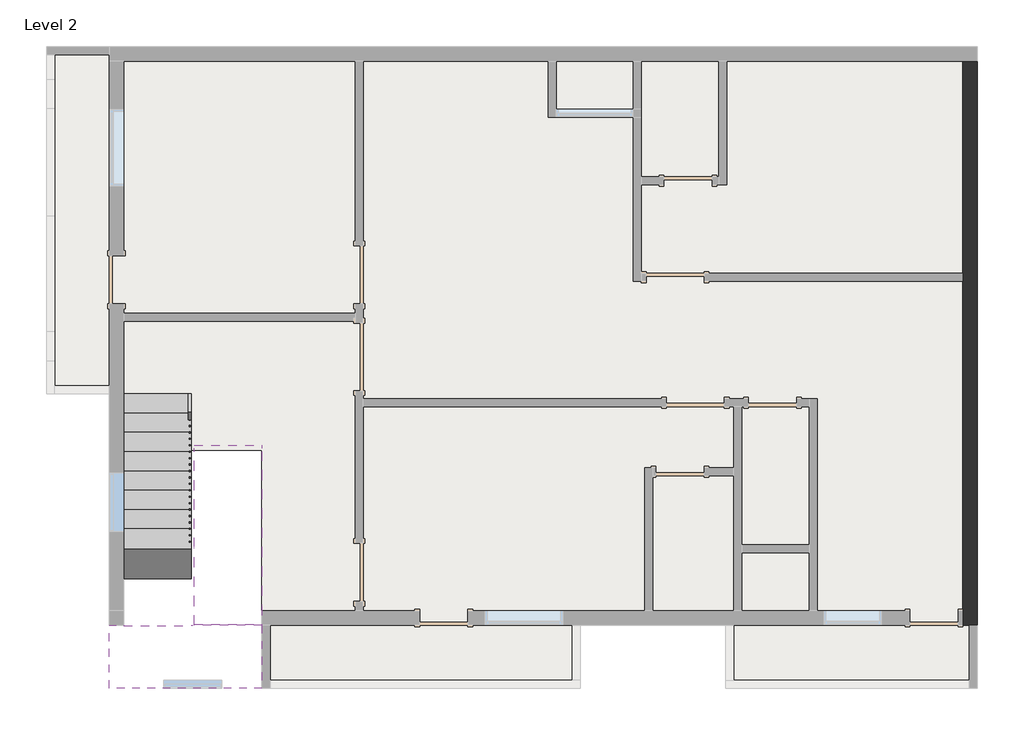
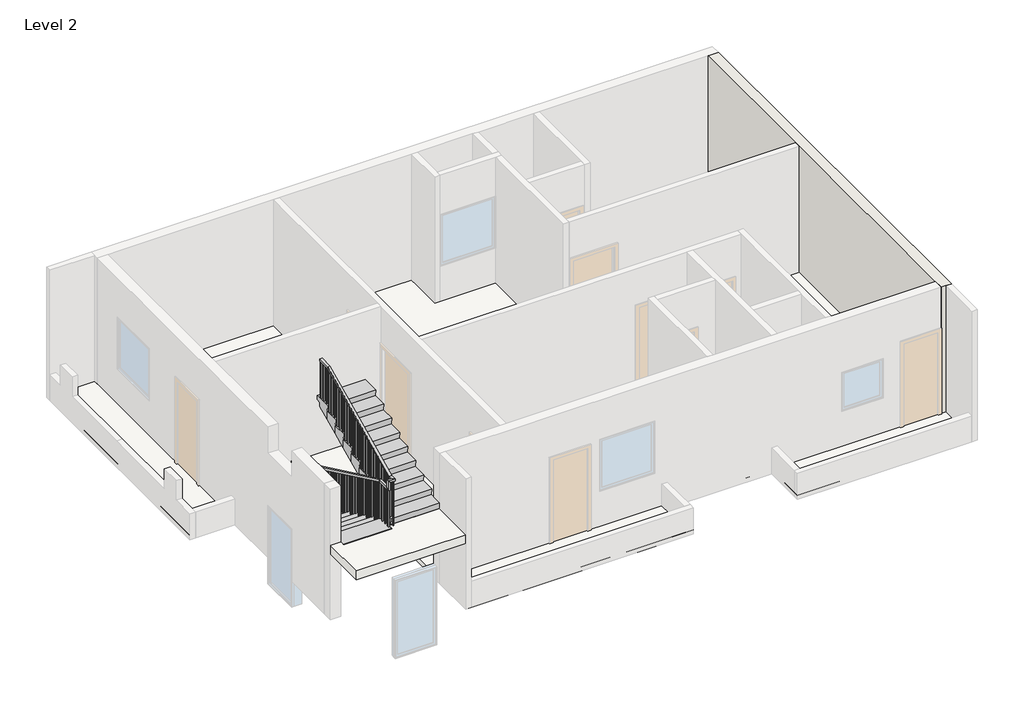
# One storey, part 2 of 2: 2 stair flights, 1 railing, 1 roof, 1 slab, 1 wall.
"""IFC4 building model written with IfcOpenShell, lengths in millimetres."""

from ifc_helpers import new_model, si_unit, frame, origin, place, context, project, spatial, polyline, outline, extrude, faceted_brep, element, save

model = new_model("IFC4")

# Units and contexts
model_context = context("Model", 3, world=origin())
ifc_project = project(units=[si_unit("LENGTHUNIT", "METRE", prefix="MILLI")], contexts=[model_context])

# Site, building, storey
site = spatial("IfcSite", under=ifc_project)
building = spatial("IfcBuilding", under=site)
storey = spatial("IfcBuildingStorey", under=building, Name="Level 2", Elevation=3048.0)

# Railing
placement = place(None, origin())
element("IfcRailing", 1, ObjectType="Handrail - Rectangular", at=placement, inside=storey, context=model_context, shape_type="SolidModel", body=[
    faceted_brep([(-9046.3394758, 7288.0495492, 4107.5428571), (-9046.3394758, 7288.0495492, 4051.2772447), (-9097.1394758, 7288.0495492, 4051.2772447), (-9097.1394758, 7288.0495492, 4107.5428571), (-9046.3394758, 3935.2495492, 5704.1142857), (-9046.3394758, 3923.7717632, 5653.3142857), (-9097.1394758, 3923.7717632, 5653.3142857), (-9097.1394758, 3935.2495492, 5704.1142857), (-9046.3394758, 3630.4495492, 5704.1142857), (-9097.1394758, 3630.4495492, 5704.1142857), (-9097.1394758, 3579.6495492, 5653.3142857), (-9046.3394758, 3579.6495492, 5653.3142857)], [[[0, 1, 2, 3]], [[1, 0, 4, 5]], [[2, 1, 5, 6]], [[3, 2, 6, 7]], [[0, 3, 7, 4]], [[8, 9, 10, 11]], [[5, 4, 8, 11]], [[6, 5, 11, 10]], [[7, 6, 10, 9]], [[4, 7, 9, 8]]]),
    faceted_brep([(-9046.3394758, 3630.4495492, 5704.1142857), (-9046.3394758, 3579.6495492, 5653.3142857), (-9097.1394758, 3579.6495492, 5653.3142857), (-9097.1394758, 3630.4495492, 5704.1142857), (-9046.3394758, 3630.4495492, 5834.7428571), (-9097.1394758, 3630.4495492, 5885.5428571), (-9097.1394758, 3579.6495492, 5885.5428571), (-9046.3394758, 3579.6495492, 5834.7428571)], [[[0, 1, 2, 3]], [[4, 5, 6, 7]], [[1, 0, 4, 7]], [[2, 1, 7, 6]], [[3, 2, 6, 5]], [[0, 3, 5, 4]]]),
    faceted_brep([(-9097.1394758, 3630.4495492, 5885.5428571), (-9046.3394758, 3630.4495492, 5834.7428571), (-9046.3394758, 3579.6495492, 5834.7428571), (-9097.1394758, 3579.6495492, 5885.5428571), (-8995.5394758, 3630.4495492, 5885.5428571), (-8995.5394758, 3630.4495492, 5834.7428571), (-8944.7394758, 3579.6495492, 5834.7428571), (-8944.7394758, 3579.6495492, 5885.5428571), (-8995.5394758, 3706.6495492, 5885.5428571), (-8995.5394758, 3718.1273353, 5834.7428571), (-8944.7394758, 3718.1273353, 5834.7428571), (-8944.7394758, 3706.6495492, 5885.5428571), (-8995.5394758, 6068.8495492, 7010.4), (-8995.5394758, 6080.3273353, 6959.6), (-8944.7394758, 6080.3273353, 6959.6), (-8944.7394758, 6068.8495492, 7010.4), (-8995.5394758, 6373.6495492, 7010.4), (-8944.7394758, 6373.6495492, 7010.4), (-8944.7394758, 6373.6495492, 6959.6), (-8995.5394758, 6373.6495492, 6959.6)], [[[0, 1, 2, 3]], [[1, 0, 4, 5]], [[2, 1, 5, 6]], [[3, 2, 6, 7]], [[0, 3, 7, 4]], [[5, 4, 8, 9]], [[6, 5, 9, 10]], [[7, 6, 10, 11]], [[4, 7, 11, 8]], [[9, 8, 12, 13]], [[10, 9, 13, 14]], [[11, 10, 14, 15]], [[8, 11, 15, 12]], [[16, 17, 18, 19]], [[13, 12, 16, 19]], [[14, 13, 19, 18]], [[15, 14, 18, 17]], [[12, 15, 17, 16]]]),
    extrude(outline(polyline([(-8979.6644758, 6338.7245492), (-8979.6644758, 6357.7745492), (-8960.6144758, 6357.7745492), (-8960.6144758, 6338.7245492), (-8979.6644758, 6338.7245492)])), frame((0.0, 0.0, 6096.0), z_axis=(0.0, 0.0, 1.0), x_axis=(1.0, 0.0, 0.0)), (0.0, 0.0, 1.0), 863.6),
    extrude(outline(polyline([(-8979.6644758, 6237.1245492), (-8979.6644758, 6256.1745492), (-8960.6144758, 6256.1745492), (-8960.6144758, 6237.1245492), (-8979.6644758, 6237.1245492)])), frame((0.0, 0.0, 6096.0), z_axis=(0.0, 0.0, 1.0), x_axis=(1.0, 0.0, 0.0)), (0.0, 0.0, 1.0), 863.6),
    extrude(outline(polyline([(-8979.6644758, 6135.5245492), (-8979.6644758, 6154.5745492), (-8960.6144758, 6154.5745492), (-8960.6144758, 6135.5245492), (-8979.6644758, 6135.5245492)])), frame((0.0, 0.0, 6096.0), z_axis=(0.0, 0.0, 1.0), x_axis=(1.0, 0.0, 0.0)), (0.0, 0.0, 1.0), 863.6),
    extrude(outline(polyline([(6052.9745492, 6946.5748638), (6052.9745492, 5950.8571429), (6033.9245492, 5950.8571429), (6033.9245492, 6937.5034352), (6052.9745492, 6946.5748638)])), frame((-8979.6644758, 0.0, 0.0), z_axis=(1.0, 0.0, 0.0), x_axis=(0.0, 1.0, 0.0)), (0.0, 0.0, 1.0), 19.05),
    extrude(outline(polyline([(5951.3745492, 6898.1939114), (5951.3745492, 5950.8571429), (5932.3245492, 5950.8571429), (5932.3245492, 6889.1224828), (5951.3745492, 6898.1939114)])), frame((-8979.6644758, 0.0, 0.0), z_axis=(1.0, 0.0, 0.0), x_axis=(0.0, 1.0, 0.0)), (0.0, 0.0, 1.0), 19.05),
    extrude(outline(polyline([(5849.7745492, 6849.812959), (5849.7745492, 5950.8571429), (5830.7245492, 5950.8571429), (5830.7245492, 6840.7415305), (5849.7745492, 6849.812959)])), frame((-8979.6644758, 0.0, 0.0), z_axis=(1.0, 0.0, 0.0), x_axis=(0.0, 1.0, 0.0)), (0.0, 0.0, 1.0), 19.05),
    extrude(outline(polyline([(5748.1745492, 6801.4320067), (5748.1745492, 5805.7142857), (5729.1245492, 5805.7142857), (5729.1245492, 6792.3605781), (5748.1745492, 6801.4320067)])), frame((-8979.6644758, 0.0, 0.0), z_axis=(1.0, 0.0, 0.0), x_axis=(0.0, 1.0, 0.0)), (0.0, 0.0, 1.0), 19.05),
    extrude(outline(polyline([(5646.5745492, 6753.0510543), (5646.5745492, 5805.7142857), (5627.5245492, 5805.7142857), (5627.5245492, 6743.9796257), (5646.5745492, 6753.0510543)])), frame((-8979.6644758, 0.0, 0.0), z_axis=(1.0, 0.0, 0.0), x_axis=(0.0, 1.0, 0.0)), (0.0, 0.0, 1.0), 19.05),
    extrude(outline(polyline([(5544.9745492, 6704.6701019), (5544.9745492, 5805.7142857), (5525.9245492, 5805.7142857), (5525.9245492, 6695.5986733), (5544.9745492, 6704.6701019)])), frame((-8979.6644758, 0.0, 0.0), z_axis=(1.0, 0.0, 0.0), x_axis=(0.0, 1.0, 0.0)), (0.0, 0.0, 1.0), 19.05),
    extrude(outline(polyline([(5443.3745492, 6656.2891495), (5443.3745492, 5660.5714286), (5424.3245492, 5660.5714286), (5424.3245492, 6647.2177209), (5443.3745492, 6656.2891495)])), frame((-8979.6644758, 0.0, 0.0), z_axis=(1.0, 0.0, 0.0), x_axis=(0.0, 1.0, 0.0)), (0.0, 0.0, 1.0), 19.05),
    extrude(outline(polyline([(5341.7745492, 6607.9081971), (5341.7745492, 5660.5714286), (5322.7245492, 5660.5714286), (5322.7245492, 6598.8367686), (5341.7745492, 6607.9081971)])), frame((-8979.6644758, 0.0, 0.0), z_axis=(1.0, 0.0, 0.0), x_axis=(0.0, 1.0, 0.0)), (0.0, 0.0, 1.0), 19.05),
    extrude(outline(polyline([(5240.1745492, 6559.5272447), (5240.1745492, 5660.5714286), (5221.1245492, 5660.5714286), (5221.1245492, 6550.4558162), (5240.1745492, 6559.5272447)])), frame((-8979.6644758, 0.0, 0.0), z_axis=(1.0, 0.0, 0.0), x_axis=(0.0, 1.0, 0.0)), (0.0, 0.0, 1.0), 19.05),
    extrude(outline(polyline([(5138.5745492, 6511.1462924), (5138.5745492, 5515.4285714), (5119.5245492, 5515.4285714), (5119.5245492, 6502.0748638), (5138.5745492, 6511.1462924)])), frame((-8979.6644758, 0.0, 0.0), z_axis=(1.0, 0.0, 0.0), x_axis=(0.0, 1.0, 0.0)), (0.0, 0.0, 1.0), 19.05),
    extrude(outline(polyline([(5036.9745492, 6462.76534), (5036.9745492, 5515.4285714), (5017.9245492, 5515.4285714), (5017.9245492, 6453.6939114), (5036.9745492, 6462.76534)])), frame((-8979.6644758, 0.0, 0.0), z_axis=(1.0, 0.0, 0.0), x_axis=(0.0, 1.0, 0.0)), (0.0, 0.0, 1.0), 19.05),
    extrude(outline(polyline([(4935.3745492, 6414.3843876), (4935.3745492, 5515.4285714), (4916.3245492, 5515.4285714), (4916.3245492, 6405.312959), (4935.3745492, 6414.3843876)])), frame((-8979.6644758, 0.0, 0.0), z_axis=(1.0, 0.0, 0.0), x_axis=(0.0, 1.0, 0.0)), (0.0, 0.0, 1.0), 19.05),
    extrude(outline(polyline([(4833.7745492, 6366.0034352), (4833.7745492, 5370.2857143), (4814.7245492, 5370.2857143), (4814.7245492, 6356.9320067), (4833.7745492, 6366.0034352)])), frame((-8979.6644758, 0.0, 0.0), z_axis=(1.0, 0.0, 0.0), x_axis=(0.0, 1.0, 0.0)), (0.0, 0.0, 1.0), 19.05),
    extrude(outline(polyline([(4732.1745492, 6317.6224828), (4732.1745492, 5370.2857143), (4713.1245492, 5370.2857143), (4713.1245492, 6308.5510543), (4732.1745492, 6317.6224828)])), frame((-8979.6644758, 0.0, 0.0), z_axis=(1.0, 0.0, 0.0), x_axis=(0.0, 1.0, 0.0)), (0.0, 0.0, 1.0), 19.05),
    extrude(outline(polyline([(4630.5745492, 6269.2415305), (4630.5745492, 5370.2857143), (4611.5245492, 5370.2857143), (4611.5245492, 6260.1701019), (4630.5745492, 6269.2415305)])), frame((-8979.6644758, 0.0, 0.0), z_axis=(1.0, 0.0, 0.0), x_axis=(0.0, 1.0, 0.0)), (0.0, 0.0, 1.0), 19.05),
    extrude(outline(polyline([(4528.9745492, 6220.8605781), (4528.9745492, 5225.1428571), (4509.9245492, 5225.1428571), (4509.9245492, 6211.7891495), (4528.9745492, 6220.8605781)])), frame((-8979.6644758, 0.0, 0.0), z_axis=(1.0, 0.0, 0.0), x_axis=(0.0, 1.0, 0.0)), (0.0, 0.0, 1.0), 19.05),
    extrude(outline(polyline([(4427.3745492, 6172.4796257), (4427.3745492, 5225.1428571), (4408.3245492, 5225.1428571), (4408.3245492, 6163.4081971), (4427.3745492, 6172.4796257)])), frame((-8979.6644758, 0.0, 0.0), z_axis=(1.0, 0.0, 0.0), x_axis=(0.0, 1.0, 0.0)), (0.0, 0.0, 1.0), 19.05),
    extrude(outline(polyline([(4325.7745492, 6124.0986733), (4325.7745492, 5225.1428571), (4306.7245492, 5225.1428571), (4306.7245492, 6115.0272447), (4325.7745492, 6124.0986733)])), frame((-8979.6644758, 0.0, 0.0), z_axis=(1.0, 0.0, 0.0), x_axis=(0.0, 1.0, 0.0)), (0.0, 0.0, 1.0), 19.05),
    extrude(outline(polyline([(4224.1745492, 6075.7177209), (4224.1745492, 5080.0), (4205.1245492, 5080.0), (4205.1245492, 6066.6462924), (4224.1745492, 6075.7177209)])), frame((-8979.6644758, 0.0, 0.0), z_axis=(1.0, 0.0, 0.0), x_axis=(0.0, 1.0, 0.0)), (0.0, 0.0, 1.0), 19.05),
    extrude(outline(polyline([(4122.5745492, 6027.3367686), (4122.5745492, 5080.0), (4103.5245492, 5080.0), (4103.5245492, 6018.26534), (4122.5745492, 6027.3367686)])), frame((-8979.6644758, 0.0, 0.0), z_axis=(1.0, 0.0, 0.0), x_axis=(0.0, 1.0, 0.0)), (0.0, 0.0, 1.0), 19.05),
    extrude(outline(polyline([(4020.9745492, 5978.9558162), (4020.9745492, 5080.0), (4001.9245492, 5080.0), (4001.9245492, 5969.8843876), (4020.9745492, 5978.9558162)])), frame((-8979.6644758, 0.0, 0.0), z_axis=(1.0, 0.0, 0.0), x_axis=(0.0, 1.0, 0.0)), (0.0, 0.0, 1.0), 19.05),
    extrude(outline(polyline([(3919.3745492, 5930.5748638), (3919.3745492, 4934.8571429), (3900.3245492, 4934.8571429), (3900.3245492, 5921.5034352), (3919.3745492, 5930.5748638)])), frame((-8979.6644758, 0.0, 0.0), z_axis=(1.0, 0.0, 0.0), x_axis=(0.0, 1.0, 0.0)), (0.0, 0.0, 1.0), 19.05),
    extrude(outline(polyline([(3817.7745492, 5882.1939114), (3817.7745492, 4934.8571429), (3798.7245492, 4934.8571429), (3798.7245492, 5873.1224828), (3817.7745492, 5882.1939114)])), frame((-8979.6644758, 0.0, 0.0), z_axis=(1.0, 0.0, 0.0), x_axis=(0.0, 1.0, 0.0)), (0.0, 0.0, 1.0), 19.05),
    extrude(outline(polyline([(3716.1745492, 5833.812959), (3716.1745492, 4934.8571429), (3697.1245492, 4934.8571429), (3697.1245492, 5824.7415305), (3716.1745492, 5833.812959)])), frame((-8979.6644758, 0.0, 0.0), z_axis=(1.0, 0.0, 0.0), x_axis=(0.0, 1.0, 0.0)), (0.0, 0.0, 1.0), 19.05),
    extrude(outline(polyline([(-9062.2144758, 3639.9745492), (-9062.2144758, 3620.9245492), (-9081.2644758, 3620.9245492), (-9081.2644758, 3639.9745492), (-9062.2144758, 3639.9745492)])), frame((0.0, 0.0, 4789.7142857), z_axis=(0.0, 0.0, 1.0), x_axis=(1.0, 0.0, 0.0)), (0.0, 0.0, 1.0), 863.6),
    extrude(outline(polyline([(-9062.2144758, 3741.5745492), (-9062.2144758, 3722.5245492), (-9081.2644758, 3722.5245492), (-9081.2644758, 3741.5745492), (-9062.2144758, 3741.5745492)])), frame((0.0, 0.0, 4789.7142857), z_axis=(0.0, 0.0, 1.0), x_axis=(1.0, 0.0, 0.0)), (0.0, 0.0, 1.0), 863.6),
    extrude(outline(polyline([(-9062.2144758, 3843.1745492), (-9062.2144758, 3824.1245492), (-9081.2644758, 3824.1245492), (-9081.2644758, 3843.1745492), (-9062.2144758, 3843.1745492)])), frame((0.0, 0.0, 4789.7142857), z_axis=(0.0, 0.0, 1.0), x_axis=(1.0, 0.0, 0.0)), (0.0, 0.0, 1.0), 863.6),
    extrude(outline(polyline([(3944.7745492, 5643.312959), (3944.7745492, 4789.7142857), (3925.7245492, 4789.7142857), (3925.7245492, 5652.3843876), (3944.7745492, 5643.312959)])), frame((-9081.2644758, 0.0, 0.0), z_axis=(1.0, 0.0, 0.0), x_axis=(0.0, 1.0, 0.0)), (0.0, 0.0, 1.0), 19.05),
    extrude(outline(polyline([(4046.3745492, 5594.9320067), (4046.3745492, 4644.5714286), (4027.3245492, 4644.5714286), (4027.3245492, 5604.0034352), (4046.3745492, 5594.9320067)])), frame((-9081.2644758, 0.0, 0.0), z_axis=(1.0, 0.0, 0.0), x_axis=(0.0, 1.0, 0.0)), (0.0, 0.0, 1.0), 19.05),
    extrude(outline(polyline([(4147.9745492, 5546.5510543), (4147.9745492, 4644.5714286), (4128.9245492, 4644.5714286), (4128.9245492, 5555.6224828), (4147.9745492, 5546.5510543)])), frame((-9081.2644758, 0.0, 0.0), z_axis=(1.0, 0.0, 0.0), x_axis=(0.0, 1.0, 0.0)), (0.0, 0.0, 1.0), 19.05),
    extrude(outline(polyline([(4249.5745492, 5498.1701019), (4249.5745492, 4644.5714286), (4230.5245492, 4644.5714286), (4230.5245492, 5507.2415305), (4249.5745492, 5498.1701019)])), frame((-9081.2644758, 0.0, 0.0), z_axis=(1.0, 0.0, 0.0), x_axis=(0.0, 1.0, 0.0)), (0.0, 0.0, 1.0), 19.05),
    extrude(outline(polyline([(4351.1745492, 5449.7891495), (4351.1745492, 4499.4285714), (4332.1245492, 4499.4285714), (4332.1245492, 5458.8605781), (4351.1745492, 5449.7891495)])), frame((-9081.2644758, 0.0, 0.0), z_axis=(1.0, 0.0, 0.0), x_axis=(0.0, 1.0, 0.0)), (0.0, 0.0, 1.0), 19.05),
    extrude(outline(polyline([(4452.7745492, 5401.4081971), (4452.7745492, 4499.4285714), (4433.7245492, 4499.4285714), (4433.7245492, 5410.4796257), (4452.7745492, 5401.4081971)])), frame((-9081.2644758, 0.0, 0.0), z_axis=(1.0, 0.0, 0.0), x_axis=(0.0, 1.0, 0.0)), (0.0, 0.0, 1.0), 19.05),
    extrude(outline(polyline([(4554.3745492, 5353.0272447), (4554.3745492, 4499.4285714), (4535.3245492, 4499.4285714), (4535.3245492, 5362.0986733), (4554.3745492, 5353.0272447)])), frame((-9081.2644758, 0.0, 0.0), z_axis=(1.0, 0.0, 0.0), x_axis=(0.0, 1.0, 0.0)), (0.0, 0.0, 1.0), 19.05),
    extrude(outline(polyline([(4655.9745492, 5304.6462924), (4655.9745492, 4354.2857143), (4636.9245492, 4354.2857143), (4636.9245492, 5313.7177209), (4655.9745492, 5304.6462924)])), frame((-9081.2644758, 0.0, 0.0), z_axis=(1.0, 0.0, 0.0), x_axis=(0.0, 1.0, 0.0)), (0.0, 0.0, 1.0), 19.05),
    extrude(outline(polyline([(4757.5745492, 5256.26534), (4757.5745492, 4354.2857143), (4738.5245492, 4354.2857143), (4738.5245492, 5265.3367686), (4757.5745492, 5256.26534)])), frame((-9081.2644758, 0.0, 0.0), z_axis=(1.0, 0.0, 0.0), x_axis=(0.0, 1.0, 0.0)), (0.0, 0.0, 1.0), 19.05),
    extrude(outline(polyline([(4859.1745492, 5207.8843876), (4859.1745492, 4354.2857143), (4840.1245492, 4354.2857143), (4840.1245492, 5216.9558162), (4859.1745492, 5207.8843876)])), frame((-9081.2644758, 0.0, 0.0), z_axis=(1.0, 0.0, 0.0), x_axis=(0.0, 1.0, 0.0)), (0.0, 0.0, 1.0), 19.05),
    extrude(outline(polyline([(4960.7745492, 5159.5034352), (4960.7745492, 4209.1428571), (4941.7245492, 4209.1428571), (4941.7245492, 5168.5748638), (4960.7745492, 5159.5034352)])), frame((-9081.2644758, 0.0, 0.0), z_axis=(1.0, 0.0, 0.0), x_axis=(0.0, 1.0, 0.0)), (0.0, 0.0, 1.0), 19.05),
    extrude(outline(polyline([(5062.3745492, 5111.1224828), (5062.3745492, 4209.1428571), (5043.3245492, 4209.1428571), (5043.3245492, 5120.1939114), (5062.3745492, 5111.1224828)])), frame((-9081.2644758, 0.0, 0.0), z_axis=(1.0, 0.0, 0.0), x_axis=(0.0, 1.0, 0.0)), (0.0, 0.0, 1.0), 19.05),
    extrude(outline(polyline([(5163.9745492, 5062.7415305), (5163.9745492, 4209.1428571), (5144.9245492, 4209.1428571), (5144.9245492, 5071.812959), (5163.9745492, 5062.7415305)])), frame((-9081.2644758, 0.0, 0.0), z_axis=(1.0, 0.0, 0.0), x_axis=(0.0, 1.0, 0.0)), (0.0, 0.0, 1.0), 19.05),
    extrude(outline(polyline([(5265.5745492, 5014.3605781), (5265.5745492, 4064.0), (5246.5245492, 4064.0), (5246.5245492, 5023.4320067), (5265.5745492, 5014.3605781)])), frame((-9081.2644758, 0.0, 0.0), z_axis=(1.0, 0.0, 0.0), x_axis=(0.0, 1.0, 0.0)), (0.0, 0.0, 1.0), 19.05),
    extrude(outline(polyline([(5367.1745492, 4965.9796257), (5367.1745492, 4064.0), (5348.1245492, 4064.0), (5348.1245492, 4975.0510543), (5367.1745492, 4965.9796257)])), frame((-9081.2644758, 0.0, 0.0), z_axis=(1.0, 0.0, 0.0), x_axis=(0.0, 1.0, 0.0)), (0.0, 0.0, 1.0), 19.05),
    extrude(outline(polyline([(5468.7745492, 4917.5986733), (5468.7745492, 4064.0), (5449.7245492, 4064.0), (5449.7245492, 4926.6701019), (5468.7745492, 4917.5986733)])), frame((-9081.2644758, 0.0, 0.0), z_axis=(1.0, 0.0, 0.0), x_axis=(0.0, 1.0, 0.0)), (0.0, 0.0, 1.0), 19.05),
    extrude(outline(polyline([(5570.3745492, 4869.2177209), (5570.3745492, 3918.8571429), (5551.3245492, 3918.8571429), (5551.3245492, 4878.2891495), (5570.3745492, 4869.2177209)])), frame((-9081.2644758, 0.0, 0.0), z_axis=(1.0, 0.0, 0.0), x_axis=(0.0, 1.0, 0.0)), (0.0, 0.0, 1.0), 19.05),
    extrude(outline(polyline([(5671.9745492, 4820.8367686), (5671.9745492, 3918.8571429), (5652.9245492, 3918.8571429), (5652.9245492, 4829.9081971), (5671.9745492, 4820.8367686)])), frame((-9081.2644758, 0.0, 0.0), z_axis=(1.0, 0.0, 0.0), x_axis=(0.0, 1.0, 0.0)), (0.0, 0.0, 1.0), 19.05),
    extrude(outline(polyline([(5773.5745492, 4772.4558162), (5773.5745492, 3918.8571429), (5754.5245492, 3918.8571429), (5754.5245492, 4781.5272447), (5773.5745492, 4772.4558162)])), frame((-9081.2644758, 0.0, 0.0), z_axis=(1.0, 0.0, 0.0), x_axis=(0.0, 1.0, 0.0)), (0.0, 0.0, 1.0), 19.05),
    extrude(outline(polyline([(5875.1745492, 4724.0748638), (5875.1745492, 3773.7142857), (5856.1245492, 3773.7142857), (5856.1245492, 4733.1462924), (5875.1745492, 4724.0748638)])), frame((-9081.2644758, 0.0, 0.0), z_axis=(1.0, 0.0, 0.0), x_axis=(0.0, 1.0, 0.0)), (0.0, 0.0, 1.0), 19.05),
    extrude(outline(polyline([(5976.7745492, 4675.6939114), (5976.7745492, 3773.7142857), (5957.7245492, 3773.7142857), (5957.7245492, 4684.76534), (5976.7745492, 4675.6939114)])), frame((-9081.2644758, 0.0, 0.0), z_axis=(1.0, 0.0, 0.0), x_axis=(0.0, 1.0, 0.0)), (0.0, 0.0, 1.0), 19.05),
    extrude(outline(polyline([(6078.3745492, 4627.312959), (6078.3745492, 3773.7142857), (6059.3245492, 3773.7142857), (6059.3245492, 4636.3843876), (6078.3745492, 4627.312959)])), frame((-9081.2644758, 0.0, 0.0), z_axis=(1.0, 0.0, 0.0), x_axis=(0.0, 1.0, 0.0)), (0.0, 0.0, 1.0), 19.05),
    extrude(outline(polyline([(6179.9745492, 4578.9320067), (6179.9745492, 3628.5714286), (6160.9245492, 3628.5714286), (6160.9245492, 4588.0034352), (6179.9745492, 4578.9320067)])), frame((-9081.2644758, 0.0, 0.0), z_axis=(1.0, 0.0, 0.0), x_axis=(0.0, 1.0, 0.0)), (0.0, 0.0, 1.0), 19.05),
    extrude(outline(polyline([(6281.5745492, 4530.5510543), (6281.5745492, 3628.5714286), (6262.5245492, 3628.5714286), (6262.5245492, 4539.6224828), (6281.5745492, 4530.5510543)])), frame((-9081.2644758, 0.0, 0.0), z_axis=(1.0, 0.0, 0.0), x_axis=(0.0, 1.0, 0.0)), (0.0, 0.0, 1.0), 19.05),
    extrude(outline(polyline([(6383.1745492, 4482.1701019), (6383.1745492, 3628.5714286), (6364.1245492, 3628.5714286), (6364.1245492, 4491.2415305), (6383.1745492, 4482.1701019)])), frame((-9081.2644758, 0.0, 0.0), z_axis=(1.0, 0.0, 0.0), x_axis=(0.0, 1.0, 0.0)), (0.0, 0.0, 1.0), 19.05),
    extrude(outline(polyline([(6484.7745492, 4433.7891495), (6484.7745492, 3483.4285714), (6465.7245492, 3483.4285714), (6465.7245492, 4442.8605781), (6484.7745492, 4433.7891495)])), frame((-9081.2644758, 0.0, 0.0), z_axis=(1.0, 0.0, 0.0), x_axis=(0.0, 1.0, 0.0)), (0.0, 0.0, 1.0), 19.05),
    extrude(outline(polyline([(6586.3745492, 4385.4081971), (6586.3745492, 3483.4285714), (6567.3245492, 3483.4285714), (6567.3245492, 4394.4796257), (6586.3745492, 4385.4081971)])), frame((-9081.2644758, 0.0, 0.0), z_axis=(1.0, 0.0, 0.0), x_axis=(0.0, 1.0, 0.0)), (0.0, 0.0, 1.0), 19.05),
    extrude(outline(polyline([(6687.9745492, 4337.0272447), (6687.9745492, 3483.4285714), (6668.9245492, 3483.4285714), (6668.9245492, 4346.0986733), (6687.9745492, 4337.0272447)])), frame((-9081.2644758, 0.0, 0.0), z_axis=(1.0, 0.0, 0.0), x_axis=(0.0, 1.0, 0.0)), (0.0, 0.0, 1.0), 19.05),
    extrude(outline(polyline([(6789.5745492, 4288.6462924), (6789.5745492, 3338.2857143), (6770.5245492, 3338.2857143), (6770.5245492, 4297.7177209), (6789.5745492, 4288.6462924)])), frame((-9081.2644758, 0.0, 0.0), z_axis=(1.0, 0.0, 0.0), x_axis=(0.0, 1.0, 0.0)), (0.0, 0.0, 1.0), 19.05),
    extrude(outline(polyline([(6891.1745492, 4240.26534), (6891.1745492, 3338.2857143), (6872.1245492, 3338.2857143), (6872.1245492, 4249.3367686), (6891.1745492, 4240.26534)])), frame((-9081.2644758, 0.0, 0.0), z_axis=(1.0, 0.0, 0.0), x_axis=(0.0, 1.0, 0.0)), (0.0, 0.0, 1.0), 19.05),
    extrude(outline(polyline([(6992.7745492, 4191.8843876), (6992.7745492, 3338.2857143), (6973.7245492, 3338.2857143), (6973.7245492, 4200.9558162), (6992.7745492, 4191.8843876)])), frame((-9081.2644758, 0.0, 0.0), z_axis=(1.0, 0.0, 0.0), x_axis=(0.0, 1.0, 0.0)), (0.0, 0.0, 1.0), 19.05),
    extrude(outline(polyline([(7094.3745492, 4143.5034352), (7094.3745492, 3193.1428571), (7075.3245492, 3193.1428571), (7075.3245492, 4152.5748638), (7094.3745492, 4143.5034352)])), frame((-9081.2644758, 0.0, 0.0), z_axis=(1.0, 0.0, 0.0), x_axis=(0.0, 1.0, 0.0)), (0.0, 0.0, 1.0), 19.05),
    extrude(outline(polyline([(7195.9745492, 4095.1224828), (7195.9745492, 3193.1428571), (7176.9245492, 3193.1428571), (7176.9245492, 4104.1939114), (7195.9745492, 4095.1224828)])), frame((-9081.2644758, 0.0, 0.0), z_axis=(1.0, 0.0, 0.0), x_axis=(0.0, 1.0, 0.0)), (0.0, 0.0, 1.0), 19.05),
    extrude(outline(polyline([(-8979.6644758, 3614.5745492), (-8960.6144758, 3614.5745492), (-8960.6144758, 3595.5245492), (-8979.6644758, 3595.5245492), (-8979.6644758, 3614.5745492)])), frame((0.0, 0.0, 4789.7142857), z_axis=(0.0, 0.0, 1.0), x_axis=(1.0, 0.0, 0.0)), (0.0, 0.0, 1.0), 1045.0285714),
    extrude(outline(polyline([(-9062.2144758, 3614.5745492), (-9062.2144758, 3595.5245492), (-9081.2644758, 3595.5245492), (-9081.2644758, 3614.5745492), (-9062.2144758, 3614.5745492)])), frame((0.0, 0.0, 4789.7142857), z_axis=(0.0, 0.0, 1.0), x_axis=(1.0, 0.0, 0.0)), (0.0, 0.0, 1.0), 863.6),
    extrude(outline(polyline([(-8979.6644758, 6354.5995492), (-8979.6644758, 6373.6495492), (-8960.6144758, 6373.6495492), (-8960.6144758, 6354.5995492), (-8979.6644758, 6354.5995492)])), frame((0.0, 0.0, 6096.0), z_axis=(0.0, 0.0, 1.0), x_axis=(1.0, 0.0, 0.0)), (0.0, 0.0, 1.0), 863.6),
    extrude(outline(polyline([(7288.0495492, 4051.2772447), (7288.0495492, 3193.1428571), (7268.9995492, 3193.1428571), (7268.9995492, 4060.3486733), (7288.0495492, 4051.2772447)])), frame((-9081.2644758, 0.0, 0.0), z_axis=(1.0, 0.0, 0.0), x_axis=(0.0, 1.0, 0.0)), (0.0, 0.0, 1.0), 19.05),
])

# Roof
element("IfcRoof", 2, ObjectType="Generic - 4\"", at=placement, inside=storey, context=model_context, shape_type="SweptSolid", body=[
    extrude(outline(polyline([(3374.2605242, 2639.8495492), (-600.8394758, 2639.8495492), (-600.8394758, 3630.4495492), (-2899.5394758, 3630.4495492), (-2899.5394758, 2639.8495492), (-7928.7394758, 2639.8495492), (-7928.7394758, 6399.0495492), (-9046.3394758, 6399.0495492), (-9046.3394758, 7288.0495492), (-11332.3394758, 7288.0495492), (-11332.3394758, 12774.4495492), (3374.2605242, 12774.4495492), (3374.2605242, 2639.8495492)])), frame((0.0, 0.0, 3048.0), z_axis=(0.0, 0.0, 1.0), x_axis=(1.0, 0.0, 0.0)), (0.0, 0.0, 1.0), 101.6),
])

# Slab
element("IfcSlab", 3, ObjectType="8\" Thickness", at=placement, inside=storey, context=model_context, shape_type="Brep", body=[
    faceted_brep([(-10341.7394758, 3630.4495492, 4789.7142857), (-10341.7394758, 2639.8495492, 4789.7142857), (-7928.7394758, 2639.8495492, 4789.7142857), (-7928.7394758, 3630.4495492, 4789.7142857), (-7928.7394758, 3649.4995492, 4789.7142857), (-8995.5394758, 3649.4995492, 4789.7142857), (-8995.5394758, 3630.4495492, 4789.7142857), (-9044.7519758, 3630.4495492, 4789.7142857), (-9044.7519758, 3519.3245492, 4789.7142857), (-10114.7269758, 3519.3245492, 4789.7142857), (-10114.7269758, 3630.4495492, 4789.7142857), (-10341.7394758, 3630.4495492, 4586.5142857), (-10341.7394758, 2639.8495492, 4586.5142857), (-7928.7394758, 2639.8495492, 4586.5142857), (-10114.7269758, 3630.4495492, 4586.5142857), (-10114.7269758, 3620.9245492, 4586.5142857), (-9044.7519758, 3620.9245492, 4586.5142857), (-9044.7519758, 3630.4495492, 4586.5142857), (-8995.5394758, 3630.4495492, 4586.5142857), (-8995.5394758, 3649.4995492, 4586.5142857), (-7928.7394758, 3649.4995492, 4586.5142857), (-7928.7394758, 3630.4495492, 4586.5142857), (-10114.7269758, 3519.3245492, 4678.5892857), (-9044.7519758, 3519.3245492, 4678.5892857), (-9044.7519758, 3620.9245492, 4678.5892857), (-10114.7269758, 3620.9245492, 4678.5892857)], [[[0, 1, 2, 3, 4, 5, 6, 7, 8, 9, 10]], [[1, 0, 11, 12]], [[2, 1, 12, 13]], [[12, 11, 14, 15, 16, 17, 18, 19, 20, 21, 13]], [[3, 2, 13, 21]], [[5, 4, 20, 19]], [[6, 18, 17, 7]], [[22, 23, 24, 25]], [[9, 22, 25, 15, 14, 10]], [[23, 22, 9, 8]], [[23, 8, 7, 17, 16, 24]], [[25, 24, 16, 15]], [[11, 0, 10, 14]], [[4, 3, 21, 20]], [[6, 5, 19, 18]]]),
])

# Stair flights
element("IfcStairFlight", 4, ObjectType="3/4\" Nosing 6 1/2\" Depth", at=placement, inside=storey, context=model_context, shape_type="Brep", body=[
    faceted_brep([(-10113.1394758, 7288.0495492, 3193.1428571), (-9046.3394758, 7288.0495492, 3193.1428571), (-9046.3394758, 7268.9995492, 3048.0), (-10113.1394758, 7268.9995492, 3048.0), (-10113.1394758, 6964.1995492, 3193.1428571), (-9046.3394758, 6964.1995492, 3193.1428571), (-9046.3394758, 6964.1995492, 3048.0), (-10113.1394758, 6964.1995492, 3048.0), (-9046.3394758, 6983.2495492, 3338.2857143), (-10113.1394758, 6983.2495492, 3338.2857143), (-10113.1394758, 6659.3995492, 3338.2857143), (-9046.3394758, 6659.3995492, 3338.2857143), (-9046.3394758, 6659.3995492, 3155.422474), (-9046.3394758, 6884.9867446, 3048.0), (-10113.1394758, 6884.9867446, 3048.0), (-10113.1394758, 6659.3995492, 3155.422474), (-9046.3394758, 6678.4495492, 3483.4285714), (-10113.1394758, 6678.4495492, 3483.4285714), (-10113.1394758, 6354.5995492, 3483.4285714), (-9046.3394758, 6354.5995492, 3483.4285714), (-9046.3394758, 6354.5995492, 3300.5653311), (-10113.1394758, 6354.5995492, 3300.5653311), (-9046.3394758, 6373.6495492, 3628.5714286), (-10113.1394758, 6373.6495492, 3628.5714286), (-10113.1394758, 6049.7995492, 3628.5714286), (-9046.3394758, 6049.7995492, 3628.5714286), (-9046.3394758, 6049.7995492, 3445.7081883), (-10113.1394758, 6049.7995492, 3445.7081883), (-9046.3394758, 6068.8495492, 3773.7142857), (-10113.1394758, 6068.8495492, 3773.7142857), (-10113.1394758, 5744.9995492, 3773.7142857), (-9046.3394758, 5744.9995492, 3773.7142857), (-9046.3394758, 5744.9995492, 3590.8510454), (-10113.1394758, 5744.9995492, 3590.8510454), (-9046.3394758, 5764.0495492, 3918.8571429), (-10113.1394758, 5764.0495492, 3918.8571429), (-10113.1394758, 5440.1995492, 3918.8571429), (-9046.3394758, 5440.1995492, 3918.8571429), (-9046.3394758, 5440.1995492, 3735.9939026), (-10113.1394758, 5440.1995492, 3735.9939026), (-9046.3394758, 5459.2495492, 4064.0), (-10113.1394758, 5459.2495492, 4064.0), (-10113.1394758, 5135.3995492, 4064.0), (-9046.3394758, 5135.3995492, 4064.0), (-9046.3394758, 5135.3995492, 3881.1367597), (-10113.1394758, 5135.3995492, 3881.1367597), (-9046.3394758, 5154.4495492, 4209.1428571), (-10113.1394758, 5154.4495492, 4209.1428571), (-10113.1394758, 4830.5995492, 4209.1428571), (-9046.3394758, 4830.5995492, 4209.1428571), (-9046.3394758, 4830.5995492, 4026.2796169), (-10113.1394758, 4830.5995492, 4026.2796169), (-9046.3394758, 4849.6495492, 4354.2857143), (-10113.1394758, 4849.6495492, 4354.2857143), (-10113.1394758, 4525.7995492, 4354.2857143), (-9046.3394758, 4525.7995492, 4354.2857143), (-9046.3394758, 4525.7995492, 4171.422474), (-10113.1394758, 4525.7995492, 4171.422474), (-9046.3394758, 4544.8495492, 4499.4285714), (-10113.1394758, 4544.8495492, 4499.4285714), (-10113.1394758, 4220.9995492, 4499.4285714), (-9046.3394758, 4220.9995492, 4499.4285714), (-9046.3394758, 4220.9995492, 4316.5653311), (-10113.1394758, 4220.9995492, 4316.5653311), (-9046.3394758, 4240.0495492, 4644.5714286), (-10113.1394758, 4240.0495492, 4644.5714286), (-10113.1394758, 3916.1995492, 4644.5714286), (-9046.3394758, 3916.1995492, 4644.5714286), (-9046.3394758, 3916.1995492, 4461.7081883), (-10113.1394758, 3916.1995492, 4461.7081883), (-9046.3394758, 3935.2495492, 4789.7142857), (-10113.1394758, 3935.2495492, 4789.7142857), (-10113.1394758, 3528.8495492, 4789.7142857), (-9046.3394758, 3528.8495492, 4789.7142857), (-9046.3394758, 3528.8495492, 4688.1142857), (-9046.3394758, 3630.4495492, 4688.1142857), (-9046.3394758, 3630.4495492, 4586.5142857), (-9046.3394758, 3654.1067446, 4586.5142857), (-10113.1394758, 3654.1067446, 4586.5142857), (-10113.1394758, 3630.4495492, 4586.5142857), (-10113.1394758, 3630.4495492, 4688.1142857), (-10113.1394758, 3528.8495492, 4688.1142857)], [[[0, 1, 2, 3]], [[1, 0, 4, 5]], [[1, 5, 6, 2]], [[4, 0, 3, 7]], [[8, 9, 10, 11]], [[6, 5, 8, 11, 12, 13]], [[4, 7, 14, 15, 10, 9]], [[5, 4, 9, 8]], [[16, 17, 18, 19]], [[16, 19, 20, 12, 11]], [[18, 17, 10, 15, 21]], [[11, 10, 17, 16]], [[22, 23, 24, 25]], [[22, 25, 26, 20, 19]], [[24, 23, 18, 21, 27]], [[19, 18, 23, 22]], [[28, 29, 30, 31]], [[28, 31, 32, 26, 25]], [[30, 29, 24, 27, 33]], [[25, 24, 29, 28]], [[34, 35, 36, 37]], [[34, 37, 38, 32, 31]], [[36, 35, 30, 33, 39]], [[31, 30, 35, 34]], [[40, 41, 42, 43]], [[40, 43, 44, 38, 37]], [[42, 41, 36, 39, 45]], [[37, 36, 41, 40]], [[46, 47, 48, 49]], [[46, 49, 50, 44, 43]], [[48, 47, 42, 45, 51]], [[43, 42, 47, 46]], [[52, 53, 54, 55]], [[52, 55, 56, 50, 49]], [[54, 53, 48, 51, 57]], [[49, 48, 53, 52]], [[58, 59, 60, 61]], [[58, 61, 62, 56, 55]], [[60, 59, 54, 57, 63]], [[55, 54, 59, 58]], [[64, 65, 66, 67]], [[64, 67, 68, 62, 61]], [[66, 65, 60, 63, 69]], [[61, 60, 65, 64]], [[70, 71, 72, 73]], [[67, 70, 73, 74, 75, 76, 77, 68]], [[72, 71, 66, 69, 78, 79, 80, 81]], [[79, 76, 75, 80]], [[67, 66, 71, 70]], [[2, 6, 13, 14, 7, 3]], [[77, 78, 69, 63, 57, 51, 45, 39, 33, 27, 21, 15, 14, 13, 12, 20, 26, 32, 38, 44, 50, 56, 62, 68]], [[81, 80, 75, 74]], [[81, 74, 73, 72]], [[78, 77, 76, 79]]]),
])
element("IfcStairFlight", 5, ObjectType="3/4\" Nosing 6 1/2\" Depth", at=placement, inside=storey, context=model_context, shape_type="Brep", body=[
    faceted_brep([(-7928.7394758, 3630.4495492, 4934.8571429), (-8995.5394758, 3630.4495492, 4934.8571429), (-8995.5394758, 3649.4995492, 4789.7142857), (-7928.7394758, 3649.4995492, 4789.7142857), (-7928.7394758, 3954.2995492, 4934.8571429), (-8995.5394758, 3954.2995492, 4934.8571429), (-8995.5394758, 3954.2995492, 4751.9939026), (-8995.5394758, 3649.4995492, 4606.8510454), (-7928.7394758, 3649.4995492, 4606.8510454), (-7928.7394758, 3954.2995492, 4751.9939026), (-8995.5394758, 3935.2495492, 5080.0), (-7928.7394758, 3935.2495492, 5080.0), (-7928.7394758, 4259.0995492, 5080.0), (-8995.5394758, 4259.0995492, 5080.0), (-8995.5394758, 4259.0995492, 4897.1367597), (-7928.7394758, 4259.0995492, 4897.1367597), (-8995.5394758, 4240.0495492, 5225.1428571), (-7928.7394758, 4240.0495492, 5225.1428571), (-7928.7394758, 4563.8995492, 5225.1428571), (-8995.5394758, 4563.8995492, 5225.1428571), (-8995.5394758, 4563.8995492, 5042.2796169), (-7928.7394758, 4563.8995492, 5042.2796169), (-8995.5394758, 4544.8495492, 5370.2857143), (-7928.7394758, 4544.8495492, 5370.2857143), (-7928.7394758, 4868.6995492, 5370.2857143), (-8995.5394758, 4868.6995492, 5370.2857143), (-8995.5394758, 4868.6995492, 5187.422474), (-7928.7394758, 4868.6995492, 5187.422474), (-8995.5394758, 4849.6495492, 5515.4285714), (-7928.7394758, 4849.6495492, 5515.4285714), (-7928.7394758, 5173.4995492, 5515.4285714), (-8995.5394758, 5173.4995492, 5515.4285714), (-8995.5394758, 5173.4995492, 5332.5653311), (-7928.7394758, 5173.4995492, 5332.5653311), (-8995.5394758, 5154.4495492, 5660.5714286), (-7928.7394758, 5154.4495492, 5660.5714286), (-7928.7394758, 5478.2995492, 5660.5714286), (-8995.5394758, 5478.2995492, 5660.5714286), (-8995.5394758, 5478.2995492, 5477.7081883), (-7928.7394758, 5478.2995492, 5477.7081883), (-8995.5394758, 5459.2495492, 5805.7142857), (-7928.7394758, 5459.2495492, 5805.7142857), (-7928.7394758, 5783.0995492, 5805.7142857), (-8995.5394758, 5783.0995492, 5805.7142857), (-8995.5394758, 5783.0995492, 5622.8510454), (-7928.7394758, 5783.0995492, 5622.8510454), (-8995.5394758, 5764.0495492, 5950.8571429), (-7928.7394758, 5764.0495492, 5950.8571429), (-7928.7394758, 6087.8995492, 5950.8571429), (-8995.5394758, 6087.8995492, 5950.8571429), (-8995.5394758, 6087.8995492, 5767.9939026), (-7928.7394758, 6087.8995492, 5767.9939026), (-8995.5394758, 6068.8495492, 6096.0), (-7928.7394758, 6068.8495492, 6096.0), (-7928.7394758, 6475.2495492, 6096.0), (-8995.5394758, 6475.2495492, 6096.0), (-8995.5394758, 6475.2495492, 5994.4), (-8995.5394758, 6373.6495492, 5994.4), (-8995.5394758, 6373.6495492, 5904.0653311), (-7928.7394758, 6373.6495492, 5904.0653311), (-7928.7394758, 6373.6495492, 5994.4), (-7928.7394758, 6475.2495492, 5994.4)], [[[0, 1, 2, 3]], [[1, 0, 4, 5]], [[1, 5, 6, 7, 2]], [[3, 2, 7, 8]], [[4, 0, 3, 8, 9]], [[10, 11, 12, 13]], [[10, 13, 14, 6, 5]], [[12, 11, 4, 9, 15]], [[11, 10, 5, 4]], [[16, 17, 18, 19]], [[16, 19, 20, 14, 13]], [[18, 17, 12, 15, 21]], [[17, 16, 13, 12]], [[22, 23, 24, 25]], [[22, 25, 26, 20, 19]], [[24, 23, 18, 21, 27]], [[23, 22, 19, 18]], [[28, 29, 30, 31]], [[28, 31, 32, 26, 25]], [[30, 29, 24, 27, 33]], [[29, 28, 25, 24]], [[34, 35, 36, 37]], [[34, 37, 38, 32, 31]], [[36, 35, 30, 33, 39]], [[35, 34, 31, 30]], [[40, 41, 42, 43]], [[40, 43, 44, 38, 37]], [[42, 41, 36, 39, 45]], [[41, 40, 37, 36]], [[46, 47, 48, 49]], [[46, 49, 50, 44, 43]], [[48, 47, 42, 45, 51]], [[47, 46, 43, 42]], [[52, 53, 54, 55]], [[52, 55, 56, 57, 58, 50, 49]], [[54, 53, 48, 51, 59, 60, 61]], [[59, 58, 57, 60]], [[53, 52, 49, 48]], [[7, 6, 14, 20, 26, 32, 38, 44, 50, 58, 59, 51, 45, 39, 33, 27, 21, 15, 9, 8]], [[61, 60, 57, 56]], [[61, 56, 55, 54]]]),
])

# Wall
element("IfcWall", 6, ObjectType="Generic - 9\"", at=placement, inside=storey, context=model_context, shape_type="Brep", body=[
    faceted_brep([(3145.6605242, 12545.8495492, 3048.0), (3145.6605242, 9193.0495492, 3048.0), (3145.6605242, 9066.0495492, 3048.0), (3145.6605242, 3859.0495492, 3048.0), (3145.6605242, 3630.4495492, 3048.0), (3145.6605242, 3630.4495492, 6096.0), (3145.6605242, 3859.0495492, 6096.0), (3145.6605242, 9066.0495492, 6096.0), (3145.6605242, 9193.0495492, 6096.0), (3145.6605242, 12545.8495492, 6096.0), (3374.2605242, 12545.8495492, 3048.0), (3374.2605242, 12545.8495492, 6096.0), (3374.2605242, 3630.4495492, 6096.0), (3374.2605242, 3630.4495492, 3048.0), (3247.2605242, 3630.4495492, 3048.0), (3247.2605242, 3630.4495492, 6096.0)], [[[0, 1, 2, 3, 4, 5, 6, 7, 8, 9]], [[10, 11, 12, 13]], [[4, 3, 2, 1, 0, 10, 13, 14]], [[9, 8, 7, 6, 5, 15, 12, 11]], [[0, 9, 11, 10]], [[5, 4, 14, 13, 12, 15]]]),
])

save(model, "model.ifc")

# Revit data of these elements
# Type "Handrail - Rectangular"
#   Assembly Code = "C2010400"
#   built-in parameter 1008612 = 0.0416667 (stored number, unit not read)
#   built-in parameter 1008611 = 0.0416667 (stored number, unit not read)
#   built-in parameter 1008609 = 0.333333 (stored number, unit not read)
#   built-in parameter 1008604 = 0.166667 (stored number, unit not read)
#   built-in parameter 1008603 = 0.166667 (stored number, unit not read)
#   Railing Height = 3' - 0"
#   built-in parameter 1008630 = 2
#   built-in parameter 1008610 = 2
#   built-in parameter 1008618 = Baluster - Square : 3/4"
# Type "Generic - 4\""
#   Assembly Code = "B1020"
#   Layers, outside or top first: 0' - 4" "01 colour 1" (function 1)
# Type "Generic - 9\""
#   Assembly Code = "B2010"
#   Layers, outside or top first: 0' - 9" no material (function 1)
# Element 1 (IfcRailing, "Handrail - Rectangular")
#   Phase Created = New Construction
# Element 2 (IfcRoof, "Generic - 4\"")
#   built-in parameter 1001705 = 10.3333 (stored number, unit not read)
#   built-in parameter 1001710 = 33615
#   Phase Created = New Construction
#   Materials on its faces: "01 colour 1"
# Element 3 (IfcSlab, "8\" Thickness")
#   Phase Created = New Construction
#   Materials on its faces: "Concrete, Cast-in-Place gray", "01 colour 1"
# Elements 4, 5 (IfcStairFlight, "3/4\" Nosing 6 1/2\" Depth")
#   Phase Created = New Construction
#   Materials on its faces: "Concrete, Cast-in-Place gray"
# Element 6 (IfcWall, "Generic - 9\"")
#   Top Offset = 0' - 0"
#   Base Offset = 0' - 0"
#   Unconnected Height = 10' - 0"
#   wall height = 10' - 0"
#   Phase Created = New Construction
#   Base Constraint = Level 2
#   Materials on its faces: "Default Wall", "02 white", "01 colour 1"
# Materials
#   "01 colour 1": class "Generic", colour RGB 120 120 120, transparency 0, Cost = 0
#   "Concrete, Cast-in-Place gray": class "Concrete", colour RGB 115 116 108, transparency 0, Description = "Cast-in-place concrete", Cost = 0
#   "Default Wall": colour RGB 80 80 80, transparency 0
#   "02 white": class "Generic", colour RGB 120 120 120, transparency 0, Cost = 0
